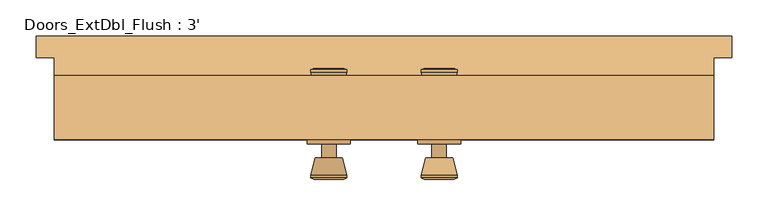
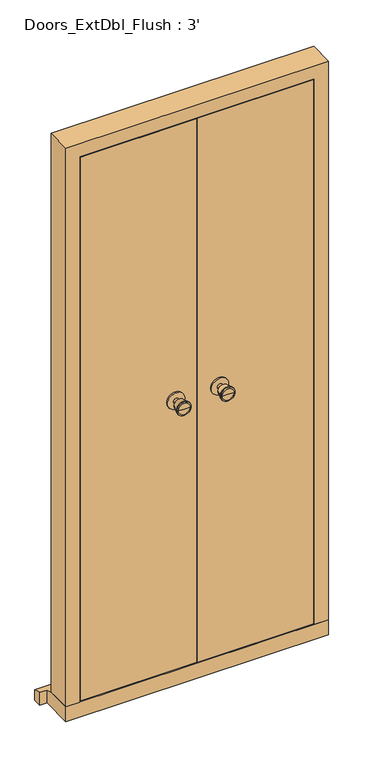
"""IFC4 building model written with IfcOpenShell, lengths in millimetres: door geometry, Doors_ExtDbl_Flush : 3'."""

from ifc_helpers import new_model, si_unit, point, frame, frame_2d, origin, place, context, project, spatial, polyline, circle_curve, trimmed, segment, composite_curve, outline, extrude, faceted_brep, source, transform, mapped, element, save
from ifc_brep_helpers import plane_surface, cylinder_surface, revolved_surface, advanced_brep


def doors_extdbl_flush_3_6b548a76(model_context):
    return source(origin(), model_context, "Body", "SolidModel", [
        advanced_brep(
        [(-76.5, -36.18, 1050.0), (-66.5, -36.18, 1050.0), (-86.5, -36.18, 1050.0), (-96.9758676, -85.18, 1050.0), (-56.0241324, -85.18, 1050.0), (-76.5, -85.18, 1050.0), (-101.5, -83.3521319, 1050.0), (-51.5, -83.3521319, 1050.0), (-101.5, -79.8884537, 1050.0), (-51.5, -79.8884537, 1050.0), (-95.136236, -55.18, 1050.0), (-57.863764, -55.18, 1050.0), (-86.5, -55.18, 1050.0), (-66.5, -55.18, 1050.0)],
        [
            (0, 1),
            (1, 2, circle_curve(frame((-76.5, -36.18, 1050.0), z_axis=(0.0, 1.0, 0.0), x_axis=(1.0, 0.0, 0.0)), 10.0)),
            (2, 0),
            (2, 1, circle_curve(frame((-76.5, -36.18, 1050.0), z_axis=(0.0, 1.0, 0.0), x_axis=(1.0, 0.0, 0.0)), 10.0)),
            (3, 4, circle_curve(frame((-76.5, -85.18, 1050.0), z_axis=(0.0, -1.0, 0.0), x_axis=(1.0, 0.0, 0.0)), 20.4758676)),
            (4, 5),
            (5, 3),
            (4, 3, circle_curve(frame((-76.5, -85.18, 1050.0), z_axis=(0.0, -1.0, 0.0), x_axis=(1.0, 0.0, 0.0)), 20.4758676)),
            (6, 7, circle_curve(frame((-76.5, -83.3521319, 1050.0), z_axis=(0.0, -1.0, 0.0), x_axis=(1.0, 0.0, 0.0)), 25.0)),
            (7, 4),
            (3, 6),
            (7, 6, circle_curve(frame((-76.5, -83.3521319, 1050.0), z_axis=(0.0, -1.0, 0.0), x_axis=(1.0, 0.0, 0.0)), 25.0)),
            (8, 9, circle_curve(frame((-76.5, -79.8884537, 1050.0), z_axis=(0.0, -1.0, 0.0), x_axis=(1.0, 0.0, 0.0)), 25.0)),
            (9, 7),
            (6, 8),
            (9, 8, circle_curve(frame((-76.5, -79.8884537, 1050.0), z_axis=(0.0, -1.0, 0.0), x_axis=(1.0, 0.0, 0.0)), 25.0)),
            (10, 11, circle_curve(frame((-76.5, -55.18, 1050.0), z_axis=(0.0, -1.0, 0.0), x_axis=(1.0, 0.0, 0.0)), 18.636236)),
            (11, 9),
            (8, 10),
            (11, 10, circle_curve(frame((-76.5, -55.18, 1050.0), z_axis=(0.0, -1.0, 0.0), x_axis=(1.0, 0.0, 0.0)), 18.636236)),
            (12, 13, circle_curve(frame((-76.5, -55.18, 1050.0), z_axis=(0.0, -1.0, 0.0), x_axis=(1.0, 0.0, 0.0)), 10.0)),
            (13, 11),
            (10, 12),
            (13, 12, circle_curve(frame((-76.5, -55.18, 1050.0), z_axis=(0.0, -1.0, 0.0), x_axis=(1.0, 0.0, 0.0)), 10.0)),
            (1, 13),
            (12, 2),
        ],
        [
            plane_surface(frame((-76.5, -36.18, 1050.0), z_axis=(0.0, 1.0, 0.0), x_axis=(1.0, 0.0, 0.0))),
            plane_surface(frame((-76.5, -85.18, 1050.0), z_axis=(0.0, -1.0, 0.0), x_axis=(1.0, 0.0, 0.0))),
            revolved_surface(polyline([(-56.0241324, -85.18, 1050.0), (-51.5, -83.3521319, 1050.0)]), (-76.5, -36.18, 1050.0), (0.0, 1.0, 0.0)),
            cylinder_surface(frame((-76.5, -36.18, 1050.0), z_axis=(0.0, 1.0, 0.0), x_axis=(1.0, 0.0, 0.0)), 25.0),
            revolved_surface(polyline([(-51.5, -79.8884537, 1050.0), (-57.863764, -55.18, 1050.0)]), (-76.5, -36.18, 1050.0), (0.0, 1.0, 0.0)),
            plane_surface(frame((-76.5, -55.18, 1050.0), z_axis=(0.0, 1.0, 0.0), x_axis=(1.0, 0.0, 0.0))),
            cylinder_surface(frame((-76.5, -36.18, 1050.0), z_axis=(0.0, 1.0, 0.0), x_axis=(1.0, 0.0, 0.0)), 10.0),
        ],
        [
            (0, [[1, 2, 3]]),
            (0, [[-3, 4, -1]]),
            (1, [[5, 6, 7]]),
            (1, [[8, -7, -6]]),
            (2, [[9, 10, -5, 11]]),
            (2, [[12, -11, -8, -10]]),
            (3, [[13, 14, -9, 15]]),
            (3, [[16, -15, -12, -14]]),
            (4, [[17, 18, -13, 19]]),
            (4, [[20, -19, -16, -18]]),
            (5, [[21, 22, -17, 23]]),
            (5, [[24, -23, -20, -22]]),
            (6, [[-2, 25, -21, 26]]),
            (6, [[-4, -26, -24, -25]]),
        ],
    ),
        extrude(outline(composite_curve([segment(trimmed(circle_curve(frame_2d((1050.0, -76.5)), 30.0), [point((1050.0, -46.5))], [point((1050.0, -106.5))], False, "CARTESIAN"), True, "CONTINUOUS"), segment(trimmed(circle_curve(frame_2d((1050.0, -76.5)), 30.0), [point((1050.0, -106.5))], [point((1050.0, -46.5))], False, "CARTESIAN"), True, "CONTINUOUS")], self_intersect=False)), frame((0.0, -36.18, 0.0), z_axis=(0.0, 1.0, 0.0), x_axis=(0.0, 0.0, 1.0)), (0.0, 0.0, 1.0), 6.0),
        advanced_brep(
        [(-76.5, 19.82, 1050.0), (-86.5, 19.82, 1050.0), (-66.5, 19.82, 1050.0), (-96.9758676, 68.82, 1050.0), (-76.5, 68.82, 1050.0), (-56.0241324, 68.82, 1050.0), (-101.5, 66.9921319, 1050.0), (-51.5, 66.9921319, 1050.0), (-101.5, 63.5284537, 1050.0), (-51.5, 63.5284537, 1050.0), (-95.136236, 38.82, 1050.0), (-57.863764, 38.82, 1050.0), (-86.5, 38.82, 1050.0), (-66.5, 38.82, 1050.0)],
        [
            (0, 1),
            (1, 2, circle_curve(frame((-76.5, 19.82, 1050.0), z_axis=(0.0, -1.0, 0.0), x_axis=(1.0, 0.0, 0.0)), 10.0)),
            (2, 0),
            (2, 1, circle_curve(frame((-76.5, 19.82, 1050.0), z_axis=(0.0, -1.0, 0.0), x_axis=(1.0, 0.0, 0.0)), 10.0)),
            (3, 4),
            (4, 5),
            (5, 3, circle_curve(frame((-76.5, 68.82, 1050.0), z_axis=(0.0, 1.0, 0.0), x_axis=(1.0, 0.0, 0.0)), 20.4758676)),
            (3, 5, circle_curve(frame((-76.5, 68.82, 1050.0), z_axis=(0.0, 1.0, 0.0), x_axis=(1.0, 0.0, 0.0)), 20.4758676)),
            (6, 3),
            (5, 7),
            (7, 6, circle_curve(frame((-76.5, 66.9921319, 1050.0), z_axis=(0.0, 1.0, 0.0), x_axis=(1.0, 0.0, 0.0)), 25.0)),
            (6, 7, circle_curve(frame((-76.5, 66.9921319, 1050.0), z_axis=(0.0, 1.0, 0.0), x_axis=(1.0, 0.0, 0.0)), 25.0)),
            (8, 6),
            (7, 9),
            (9, 8, circle_curve(frame((-76.5, 63.5284537, 1050.0), z_axis=(0.0, 1.0, 0.0), x_axis=(1.0, 0.0, 0.0)), 25.0)),
            (8, 9, circle_curve(frame((-76.5, 63.5284537, 1050.0), z_axis=(0.0, 1.0, 0.0), x_axis=(1.0, 0.0, 0.0)), 25.0)),
            (10, 8),
            (9, 11),
            (11, 10, circle_curve(frame((-76.5, 38.82, 1050.0), z_axis=(0.0, 1.0, 0.0), x_axis=(1.0, 0.0, 0.0)), 18.636236)),
            (10, 11, circle_curve(frame((-76.5, 38.82, 1050.0), z_axis=(0.0, 1.0, 0.0), x_axis=(1.0, 0.0, 0.0)), 18.636236)),
            (12, 10),
            (11, 13),
            (13, 12, circle_curve(frame((-76.5, 38.82, 1050.0), z_axis=(0.0, 1.0, 0.0), x_axis=(1.0, 0.0, 0.0)), 10.0)),
            (12, 13, circle_curve(frame((-76.5, 38.82, 1050.0), z_axis=(0.0, 1.0, 0.0), x_axis=(1.0, 0.0, 0.0)), 10.0)),
            (1, 12),
            (13, 2),
        ],
        [
            plane_surface(frame((-76.5, 19.82, 1050.0), z_axis=(0.0, -1.0, 0.0), x_axis=(1.0, 0.0, 0.0))),
            plane_surface(frame((-76.5, 68.82, 1050.0), z_axis=(0.0, 1.0, 0.0), x_axis=(1.0, 0.0, 0.0))),
            revolved_surface(polyline([(-56.0241324, 68.82, 1050.0), (-51.5, 66.9921319, 1050.0)]), (-76.5, 19.82, 1050.0), (0.0, -1.0, 0.0)),
            cylinder_surface(frame((-76.5, 19.82, 1050.0), z_axis=(0.0, -1.0, 0.0), x_axis=(1.0, 0.0, 0.0)), 25.0),
            revolved_surface(polyline([(-51.5, 63.5284537, 1050.0), (-57.863764, 38.82, 1050.0)]), (-76.5, 19.82, 1050.0), (0.0, -1.0, 0.0)),
            plane_surface(frame((-76.5, 38.82, 1050.0), z_axis=(0.0, -1.0, 0.0), x_axis=(1.0, 0.0, 0.0))),
            cylinder_surface(frame((-76.5, 19.82, 1050.0), z_axis=(0.0, -1.0, 0.0), x_axis=(1.0, 0.0, 0.0)), 10.0),
        ],
        [
            (0, [[1, 2, 3]]),
            (0, [[-3, 4, -1]]),
            (1, [[5, 6, 7]]),
            (1, [[-6, -5, 8]]),
            (2, [[9, -7, 10, 11]]),
            (2, [[-10, -8, -9, 12]]),
            (3, [[13, -11, 14, 15]]),
            (3, [[-14, -12, -13, 16]]),
            (4, [[17, -15, 18, 19]]),
            (4, [[-18, -16, -17, 20]]),
            (5, [[21, -19, 22, 23]]),
            (5, [[-22, -20, -21, 24]]),
            (6, [[25, -23, 26, -2]]),
            (6, [[-26, -24, -25, -4]]),
        ],
    ),
        extrude(outline(composite_curve([segment(trimmed(circle_curve(frame_2d((1050.0, -76.5)), 30.0), [point((1050.0, -46.5))], [point((1050.0, -106.5))], False, "CARTESIAN"), True, "CONTINUOUS"), segment(trimmed(circle_curve(frame_2d((1050.0, -76.5)), 30.0), [point((1050.0, -106.5))], [point((1050.0, -46.5))], False, "CARTESIAN"), True, "CONTINUOUS")], self_intersect=False)), frame((0.0, 13.82, 0.0), z_axis=(0.0, 1.0, 0.0), x_axis=(0.0, 0.0, 1.0)), (0.0, 0.0, 1.0), 6.0),
        advanced_brep(
        [(76.5, -36.18, 1050.0), (86.5, -36.18, 1050.0), (66.5, -36.18, 1050.0), (96.9758676, -85.18, 1050.0), (76.5, -85.18, 1050.0), (56.0241324, -85.18, 1050.0), (101.5, -83.3521319, 1050.0), (51.5, -83.3521319, 1050.0), (101.5, -79.8884537, 1050.0), (51.5, -79.8884537, 1050.0), (95.136236, -55.18, 1050.0), (57.863764, -55.18, 1050.0), (86.5, -55.18, 1050.0), (66.5, -55.18, 1050.0)],
        [
            (0, 1),
            (1, 2, circle_curve(frame((76.5, -36.18, 1050.0), z_axis=(0.0, 1.0, 0.0), x_axis=(-1.0, 0.0, 0.0)), 10.0)),
            (2, 0),
            (2, 1, circle_curve(frame((76.5, -36.18, 1050.0), z_axis=(0.0, 1.0, 0.0), x_axis=(-1.0, 0.0, 0.0)), 10.0)),
            (3, 4),
            (4, 5),
            (5, 3, circle_curve(frame((76.5, -85.18, 1050.0), z_axis=(0.0, -1.0, 0.0), x_axis=(-1.0, 0.0, 0.0)), 20.4758676)),
            (3, 5, circle_curve(frame((76.5, -85.18, 1050.0), z_axis=(0.0, -1.0, 0.0), x_axis=(-1.0, 0.0, 0.0)), 20.4758676)),
            (6, 3),
            (5, 7),
            (7, 6, circle_curve(frame((76.5, -83.3521319, 1050.0), z_axis=(0.0, -1.0, 0.0), x_axis=(-1.0, 0.0, 0.0)), 25.0)),
            (6, 7, circle_curve(frame((76.5, -83.3521319, 1050.0), z_axis=(0.0, -1.0, 0.0), x_axis=(-1.0, 0.0, 0.0)), 25.0)),
            (8, 6),
            (7, 9),
            (9, 8, circle_curve(frame((76.5, -79.8884537, 1050.0), z_axis=(0.0, -1.0, 0.0), x_axis=(-1.0, 0.0, 0.0)), 25.0)),
            (8, 9, circle_curve(frame((76.5, -79.8884537, 1050.0), z_axis=(0.0, -1.0, 0.0), x_axis=(-1.0, 0.0, 0.0)), 25.0)),
            (10, 8),
            (9, 11),
            (11, 10, circle_curve(frame((76.5, -55.18, 1050.0), z_axis=(0.0, -1.0, 0.0), x_axis=(-1.0, 0.0, 0.0)), 18.636236)),
            (10, 11, circle_curve(frame((76.5, -55.18, 1050.0), z_axis=(0.0, -1.0, 0.0), x_axis=(-1.0, 0.0, 0.0)), 18.636236)),
            (12, 10),
            (11, 13),
            (13, 12, circle_curve(frame((76.5, -55.18, 1050.0), z_axis=(0.0, -1.0, 0.0), x_axis=(-1.0, 0.0, 0.0)), 10.0)),
            (12, 13, circle_curve(frame((76.5, -55.18, 1050.0), z_axis=(0.0, -1.0, 0.0), x_axis=(-1.0, 0.0, 0.0)), 10.0)),
            (1, 12),
            (13, 2),
        ],
        [
            plane_surface(frame((76.5, -36.18, 1050.0), z_axis=(0.0, 1.0, 0.0), x_axis=(-1.0, 0.0, 0.0))),
            plane_surface(frame((76.5, -85.18, 1050.0), z_axis=(0.0, -1.0, 0.0), x_axis=(-1.0, 0.0, 0.0))),
            revolved_surface(polyline([(56.0241324, -85.18, 1050.0), (51.5, -83.3521319, 1050.0)]), (76.5, -36.18, 1050.0), (0.0, 1.0, 0.0)),
            cylinder_surface(frame((76.5, -36.18, 1050.0), z_axis=(0.0, 1.0, 0.0), x_axis=(-1.0, 0.0, 0.0)), 25.0),
            revolved_surface(polyline([(51.5, -79.8884537, 1050.0), (57.863764, -55.18, 1050.0)]), (76.5, -36.18, 1050.0), (0.0, 1.0, 0.0)),
            plane_surface(frame((76.5, -55.18, 1050.0), z_axis=(0.0, 1.0, 0.0), x_axis=(-1.0, 0.0, 0.0))),
            cylinder_surface(frame((76.5, -36.18, 1050.0), z_axis=(0.0, 1.0, 0.0), x_axis=(-1.0, 0.0, 0.0)), 10.0),
        ],
        [
            (0, [[1, 2, 3]]),
            (0, [[-3, 4, -1]]),
            (1, [[5, 6, 7]]),
            (1, [[-6, -5, 8]]),
            (2, [[9, -7, 10, 11]]),
            (2, [[-10, -8, -9, 12]]),
            (3, [[13, -11, 14, 15]]),
            (3, [[-14, -12, -13, 16]]),
            (4, [[17, -15, 18, 19]]),
            (4, [[-18, -16, -17, 20]]),
            (5, [[21, -19, 22, 23]]),
            (5, [[-22, -20, -21, 24]]),
            (6, [[25, -23, 26, -2]]),
            (6, [[-26, -24, -25, -4]]),
        ],
    ),
        extrude(outline(composite_curve([segment(trimmed(circle_curve(frame_2d((1050.0, 76.5)), 30.0), [point((1050.0, 46.5))], [point((1050.0, 106.5))], False, "CARTESIAN"), True, "CONTINUOUS"), segment(trimmed(circle_curve(frame_2d((1050.0, 76.5)), 30.0), [point((1050.0, 106.5))], [point((1050.0, 46.5))], False, "CARTESIAN"), True, "CONTINUOUS")], self_intersect=False)), frame((0.0, -36.18, 0.0), z_axis=(0.0, 1.0, 0.0), x_axis=(0.0, 0.0, 1.0)), (0.0, 0.0, 1.0), 6.0),
        advanced_brep(
        [(76.5, 19.82, 1050.0), (66.5, 19.82, 1050.0), (86.5, 19.82, 1050.0), (96.9758676, 68.82, 1050.0), (56.0241324, 68.82, 1050.0), (76.5, 68.82, 1050.0), (101.5, 66.9921319, 1050.0), (51.5, 66.9921319, 1050.0), (101.5, 63.5284537, 1050.0), (51.5, 63.5284537, 1050.0), (95.136236, 38.82, 1050.0), (57.863764, 38.82, 1050.0), (86.5, 38.82, 1050.0), (66.5, 38.82, 1050.0)],
        [
            (0, 1),
            (1, 2, circle_curve(frame((76.5, 19.82, 1050.0), z_axis=(0.0, -1.0, 0.0), x_axis=(-1.0, 0.0, 0.0)), 10.0)),
            (2, 0),
            (2, 1, circle_curve(frame((76.5, 19.82, 1050.0), z_axis=(0.0, -1.0, 0.0), x_axis=(-1.0, 0.0, 0.0)), 10.0)),
            (3, 4, circle_curve(frame((76.5, 68.82, 1050.0), z_axis=(0.0, 1.0, 0.0), x_axis=(-1.0, 0.0, 0.0)), 20.4758676)),
            (4, 5),
            (5, 3),
            (4, 3, circle_curve(frame((76.5, 68.82, 1050.0), z_axis=(0.0, 1.0, 0.0), x_axis=(-1.0, 0.0, 0.0)), 20.4758676)),
            (6, 7, circle_curve(frame((76.5, 66.9921319, 1050.0), z_axis=(0.0, 1.0, 0.0), x_axis=(-1.0, 0.0, 0.0)), 25.0)),
            (7, 4),
            (3, 6),
            (7, 6, circle_curve(frame((76.5, 66.9921319, 1050.0), z_axis=(0.0, 1.0, 0.0), x_axis=(-1.0, 0.0, 0.0)), 25.0)),
            (8, 9, circle_curve(frame((76.5, 63.5284537, 1050.0), z_axis=(0.0, 1.0, 0.0), x_axis=(-1.0, 0.0, 0.0)), 25.0)),
            (9, 7),
            (6, 8),
            (9, 8, circle_curve(frame((76.5, 63.5284537, 1050.0), z_axis=(0.0, 1.0, 0.0), x_axis=(-1.0, 0.0, 0.0)), 25.0)),
            (10, 11, circle_curve(frame((76.5, 38.82, 1050.0), z_axis=(0.0, 1.0, 0.0), x_axis=(-1.0, 0.0, 0.0)), 18.636236)),
            (11, 9),
            (8, 10),
            (11, 10, circle_curve(frame((76.5, 38.82, 1050.0), z_axis=(0.0, 1.0, 0.0), x_axis=(-1.0, 0.0, 0.0)), 18.636236)),
            (12, 13, circle_curve(frame((76.5, 38.82, 1050.0), z_axis=(0.0, 1.0, 0.0), x_axis=(-1.0, 0.0, 0.0)), 10.0)),
            (13, 11),
            (10, 12),
            (13, 12, circle_curve(frame((76.5, 38.82, 1050.0), z_axis=(0.0, 1.0, 0.0), x_axis=(-1.0, 0.0, 0.0)), 10.0)),
            (1, 13),
            (12, 2),
        ],
        [
            plane_surface(frame((76.5, 19.82, 1050.0), z_axis=(0.0, -1.0, 0.0), x_axis=(-1.0, 0.0, 0.0))),
            plane_surface(frame((76.5, 68.82, 1050.0), z_axis=(0.0, 1.0, 0.0), x_axis=(-1.0, 0.0, 0.0))),
            revolved_surface(polyline([(56.0241324, 68.82, 1050.0), (51.5, 66.9921319, 1050.0)]), (76.5, 19.82, 1050.0), (0.0, -1.0, 0.0)),
            cylinder_surface(frame((76.5, 19.82, 1050.0), z_axis=(0.0, -1.0, 0.0), x_axis=(-1.0, 0.0, 0.0)), 25.0),
            revolved_surface(polyline([(51.5, 63.5284537, 1050.0), (57.863764, 38.82, 1050.0)]), (76.5, 19.82, 1050.0), (0.0, -1.0, 0.0)),
            plane_surface(frame((76.5, 38.82, 1050.0), z_axis=(0.0, -1.0, 0.0), x_axis=(-1.0, 0.0, 0.0))),
            cylinder_surface(frame((76.5, 19.82, 1050.0), z_axis=(0.0, -1.0, 0.0), x_axis=(-1.0, 0.0, 0.0)), 10.0),
        ],
        [
            (0, [[1, 2, 3]]),
            (0, [[-3, 4, -1]]),
            (1, [[5, 6, 7]]),
            (1, [[8, -7, -6]]),
            (2, [[9, 10, -5, 11]]),
            (2, [[12, -11, -8, -10]]),
            (3, [[13, 14, -9, 15]]),
            (3, [[16, -15, -12, -14]]),
            (4, [[17, 18, -13, 19]]),
            (4, [[20, -19, -16, -18]]),
            (5, [[21, 22, -17, 23]]),
            (5, [[24, -23, -20, -22]]),
            (6, [[-2, 25, -21, 26]]),
            (6, [[-4, -26, -24, -25]]),
        ],
    ),
        extrude(outline(composite_curve([segment(trimmed(circle_curve(frame_2d((1050.0, 76.5)), 30.0), [point((1050.0, 46.5))], [point((1050.0, 106.5))], False, "CARTESIAN"), True, "CONTINUOUS"), segment(trimmed(circle_curve(frame_2d((1050.0, 76.5)), 30.0), [point((1050.0, 106.5))], [point((1050.0, 46.5))], False, "CARTESIAN"), True, "CONTINUOUS")], self_intersect=False)), frame((0.0, 13.82, 0.0), z_axis=(0.0, 1.0, 0.0), x_axis=(0.0, 0.0, 1.0)), (0.0, 0.0, 1.0), 6.0),
        faceted_brep([(386.7, 58.82, 54.5), (457.2, 58.82, 54.5), (457.2, -30.18, 54.5), (408.7, -30.18, 54.5), (408.7, 16.82, 54.5), (386.7, 16.82, 54.5), (386.7, 58.82, 2039.5), (-386.7, 58.82, 2039.5), (-386.7, 58.82, 54.5), (-457.2, 58.82, 54.5), (-457.2, 58.82, 2110.0), (457.2, 58.82, 2110.0), (457.2, -30.18, 2110.0), (-457.2, -30.18, 2110.0), (-457.2, -30.18, 54.5), (-408.7, -30.18, 54.5), (-408.7, -30.18, 2061.5), (408.7, -30.18, 2061.5), (408.7, 16.82, 2061.5), (-408.7, 16.82, 2061.5), (-408.7, 16.82, 54.5), (-386.7, 16.82, 54.5), (-386.7, 16.82, 2039.5), (386.7, 16.82, 2039.5)], [[[0, 1, 2, 3, 4, 5]], [[1, 0, 6, 7, 8, 9, 10, 11]], [[2, 1, 11, 12]], [[3, 2, 12, 13, 14, 15, 16, 17]], [[4, 3, 17, 18]], [[5, 4, 18, 19, 20, 21, 22, 23]], [[0, 5, 23, 6]], [[7, 22, 21, 8]], [[8, 21, 20, 15, 14, 9]], [[13, 10, 9, 14]], [[19, 16, 15, 20]], [[12, 11, 10, 13]], [[18, 17, 16, 19]], [[6, 23, 22, 7]]]),
        faceted_brep([(482.2, 113.82, 0.0), (482.2, 113.82, 38.5947221), (482.2, 83.82, 47.2703282), (482.2, 83.82, 0.0), (-482.2, 113.82, 38.5947221), (-482.2, 113.82, 0.0), (-482.2, 83.82, 0.0), (-482.2, 83.82, 47.2703282), (457.2, 83.82, 0.0), (457.2, -30.18, 0.0), (-457.2, -30.18, 0.0), (-457.2, 83.82, 0.0), (-457.2, 83.82, 47.2703282), (-457.2, 58.82, 54.5), (457.2, 58.82, 54.5), (457.2, 83.82, 47.2703282), (-457.2, -30.18, 54.5), (457.2, -30.18, 54.5)], [[[0, 1, 2, 3]], [[4, 5, 6, 7]], [[5, 0, 3, 8, 9, 10, 11, 6]], [[1, 0, 5, 4]], [[1, 4, 7, 12, 13, 14, 15, 2]], [[13, 16, 17, 14]], [[16, 10, 9, 17]], [[12, 11, 10, 16, 13]], [[11, 12, 7, 6]], [[8, 15, 14, 17, 9]], [[15, 8, 3, 2]]]),
        extrude(outline(polyline([(405.7, -30.18), (1.5, -30.18), (1.5, 13.82), (405.7, 13.82), (405.7, -30.18)])), frame((0.0, 0.0, 58.5), z_axis=(0.0, 0.0, 1.0), x_axis=(1.0, 0.0, 0.0)), (0.0, 0.0, 1.0), 2000.0),
        extrude(outline(polyline([(-1.5, -30.18), (-405.7, -30.18), (-405.7, 13.82), (-1.5, 13.82), (-1.5, -30.18)])), frame((0.0, 0.0, 58.5), z_axis=(0.0, 0.0, 1.0), x_axis=(1.0, 0.0, 0.0)), (0.0, 0.0, 1.0), 2000.0),
    ])


if __name__ == "__main__":
    model = new_model("IFC4")
    model_context = context("Model", 3, world=origin())
    ifc_project = project(units=[si_unit("LENGTHUNIT", "METRE", prefix="MILLI")], contexts=[model_context])
    site = spatial("IfcSite", under=ifc_project)
    building = spatial("IfcBuilding", under=site)
    placement = place(None, origin())
    doors_extdbl_flush_3_shape = doors_extdbl_flush_3_6b548a76(model_context)
    element("IfcDoor", 1, ObjectType="Doors_ExtDbl_Flush : 3'", at=placement, inside=building, context=model_context, shape_type="MappedRepresentation", body=[
        mapped(doors_extdbl_flush_3_shape, transform((0.0, 0.0, 0.0), x_axis=(1.0, 0.0, 0.0), y_axis=(0.0, 1.0, 0.0), z_axis=(0.0, 0.0, 1.0))),
    ])
    save(model, "model.ifc")

# Revit data of these elements
# Type "Doors_ExtDbl_Flush : 3'"
#   Type Mark = "55"
#   Type Comments = "External Double"
#   Operation = "DoubleDoorSingleSwing"
#   Keynote = "L20"
#   Analytic Construction = "Metal"
#   Wrap Layers (Ext) from Ext = 0.336286 ft
#   Wrap Layers (Int) from Ext = 0.582349 ft
#   Thickness = 0.144357 ft
#   Rough Width = 3.0 ft
#   Rough Height = 6.922572 ft
#   O/A Frame Width = 0.209974 ft
#   Heat Transfer Coefficient (U) = 3.7021 W/(m²·K)
#   Handle Z Distance = 3.444882 ft
#   FrameWidth = 0.137795 ft
#   FrameOffset - External = 0.082021 ft
#   FrameDepth = 0.291995 ft
#   Door Panel Width = 1.326115 ft
#   Door Panel Thickness = 0.144357 ft
#   Door Panel Height = 6.56168 ft
#   Cill Thickness = 0.178806 ft
#   Cill Projection = 0.098425 ft
#   Handle X Distance = 0.246063 ft
#   Height = 6.922572 ft
#   Structural Tolerance = 0.021325 ft
#   Tolerance = 0.009843 ft
#   Undercut = 0.013123 ft
#   Width = 3.0 ft
#   Cill Extension = 0.082021 ft
#   Cavity Closer Width = 0.164042 ft
#   Cavity Closer Offset from Ext = 0.336286 ft
#   Cavity Closer Depth = 0.278871 ft
#   Vis - Ironmongery = yes
#   Vis - Cavity Closers = yes
#   Function = 1
#   Material Door = Door - Panel
#   Material Frame = Door - Frame/Mullion
#   Material Ironmongery = Door - Handle
#   Visual Light Transmittance = 0
#   Thermal Resistance (R) = 0
#   Solar Heat Gain Coefficient = 0
#   Wall Closure = (empty or 0)
# Element 1 (IfcDoor, "Doors_ExtDbl_Flush : 3'")
#   Materials on its faces: "Door - Handle", "Door - Frame/Mullion", "Door - Panel"
# Materials
#   "Door - Panel": class "Wood", colour RGB 210 159 95, transparency 0, Keynote = "L20", Cost = 0
#   "Door - Frame/Mullion": class "Wood", colour RGB 212 179 113, transparency 0, Keynote = "L20", Cost = 0
#   "Door - Handle": colour RGB 0 0 0, transparency 0, Keynote = "P21", Cost = 0
